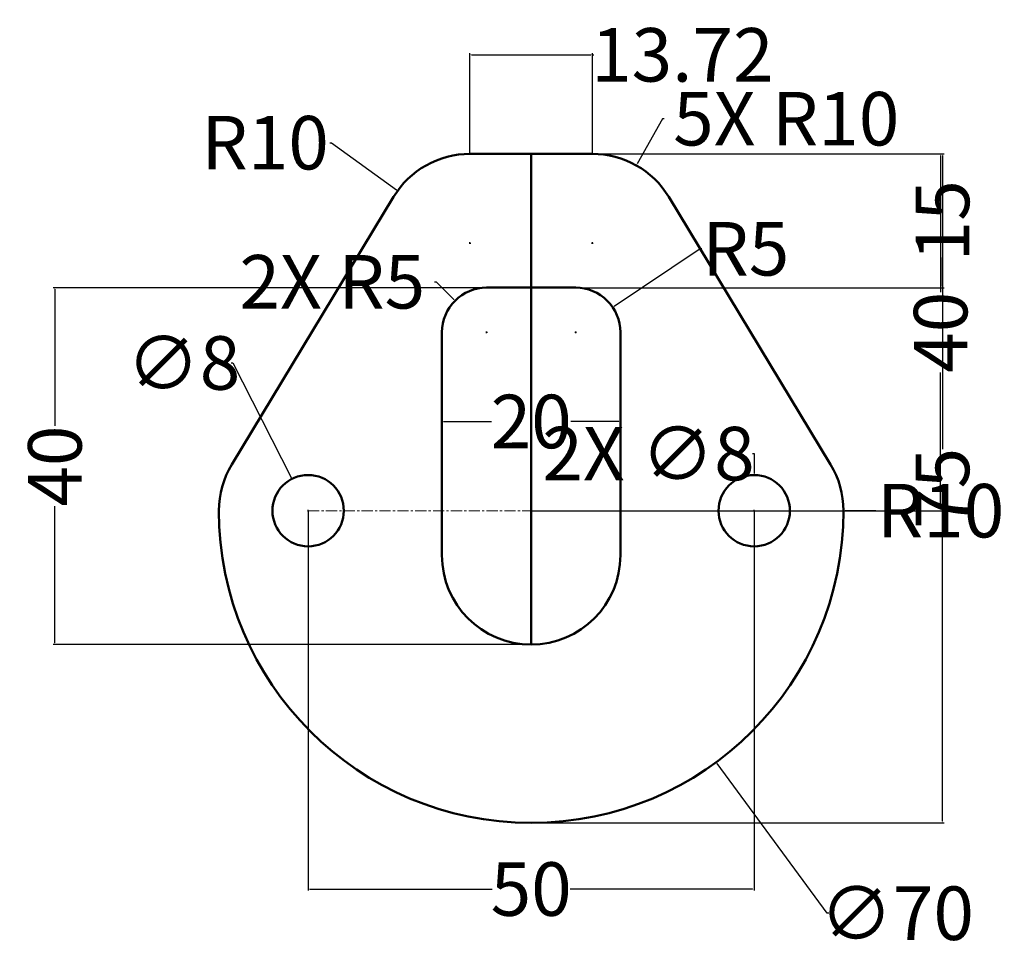
# Model space of a CAD drawing. Units: millimetres. Extents: x 6 to 117, y 2 to 106.
import ezdxf

# ---------------------------------------------------------------- set-up
doc = ezdxf.new("R2010")
doc.units = ezdxf.units.MM
doc.header["$MEASUREMENT"] = 0
doc.linetypes.add('CENTER', pattern=[2, 1.25, -0.25, 0.25, -0.25])
for name, color, linetype, lineweight in [('M-CNTR', 4, 'CENTER', 18), ('M-DIMS', 2, 'Continuous', 25), ('M-OUTL', 7, 'Continuous', 50)]:
    doc.layers.add(name, color=color, linetype=linetype, lineweight=lineweight)
doc.styles.get("Standard").update_dxf_attribs({"font": 'arial.ttf'})
doc.dimstyles.get("Standard").update_dxf_attribs({"dimtxt": 6, "dimasz": 0.18, "dimexe": 0.18, "dimexo": 0.0625, "dimgap": 0.09, "dimtad": 0, "dimtoh": 1, "dimdec": 0, "dimzin": 0, "dimdsep": 46, "dimtxsty": 'Standard', "dimcen": 0.09, "dimadec": 0, "dimazin": 0, "dimtfac": 1, "dimtdec": 0, "dimtofl": 0, "dimtmove": 0, "dimatfit": 3, "dimfxl": 1, "dimtolj": 1, "dimtzin": 0, "dimarcsym": 0})

# ---------------------------------------------------------------- blocks, each defined once
blk = doc.blocks.new('*D1')
at = {"layer": 'Defpoints', "color": 0, "transparency": 16777216}
for p in [(38.77, 50.96), (88.77, 50.96), (88.77, 8.55)]:
    blk.add_point(p, dxfattribs=at)
at = {"layer": 'M-DIMS', "color": 0, "lineweight": -2, "transparency": 16777216}
for p, q in [((38.77, 50.9), (38.77, 8.37)), ((88.77, 50.9), (88.77, 8.37)), ((38.95, 8.55), (59.39, 8.55)), ((88.59, 8.55), (68.15, 8.55))]:
    blk.add_line(p, q, dxfattribs=at)
at = {"layer": 'M-DIMS', "color": 0, "transparency": 16777216}
for points in [[(38.95, 8.58), (38.95, 8.52), (38.77, 8.55)], [(88.59, 8.58), (88.59, 8.52), (88.77, 8.55)]]:
    blk.add_solid(points, dxfattribs=at)
at = {"layer": 'M-DIMS', "color": 0, "transparency": 16777216, "insert": (63.77, 8.55), "char_height": 6, "attachment_point": 5}
blk.add_mtext('\\A1;50', dxfattribs=at)
blk = doc.blocks.new('*D2')
at = {"layer": 'Defpoints', "color": 0, "transparency": 16777216}
for p in [(63.77, 75.96), (10.38, 35.96), (63.77, 35.96)]:
    blk.add_point(p, dxfattribs=at)
at = {"layer": 'M-DIMS', "color": 0, "lineweight": -2, "transparency": 16777216}
for p, q in [((63.71, 75.96), (10.2, 75.96)), ((10.38, 75.78), (10.38, 60.46)), ((10.38, 36.14), (10.38, 51.46)), ((63.71, 35.96), (10.2, 35.96))]:
    blk.add_line(p, q, dxfattribs=at)
at = {"layer": 'M-DIMS', "color": 0, "transparency": 16777216}
for points in [[(10.35, 75.78), (10.41, 75.78), (10.38, 75.96)], [(10.35, 36.14), (10.41, 36.14), (10.38, 35.96)]]:
    blk.add_solid(points, dxfattribs=at)
at = {"layer": 'M-DIMS', "color": 0, "transparency": 16777216, "insert": (10.38, 55.96), "char_height": 6, "attachment_point": 5, "rotation": 90}
blk.add_mtext('\\A1;40', dxfattribs=at)
blk = doc.blocks.new('*D3')
at = {"layer": 'Defpoints', "color": 0, "transparency": 16777216}
for p in [(63.77, 90.96), (109.66, 90.96), (63.77, 50.96)]:
    blk.add_point(p, dxfattribs=at)
at = {"layer": 'M-DIMS', "color": 0, "lineweight": -2, "transparency": 16777216}
for p, q in [((63.83, 90.96), (109.84, 90.96)), ((109.66, 90.78), (109.66, 75.46)), ((109.66, 51.14), (109.66, 66.46)), ((63.83, 50.96), (109.84, 50.96))]:
    blk.add_line(p, q, dxfattribs=at)
at = {"layer": 'M-DIMS', "color": 0, "transparency": 16777216}
for points in [[(109.63, 90.78), (109.69, 90.78), (109.66, 90.96)], [(109.63, 51.14), (109.69, 51.14), (109.66, 50.96)]]:
    blk.add_solid(points, dxfattribs=at)
at = {"layer": 'M-DIMS', "color": 0, "transparency": 16777216, "insert": (109.66, 70.96), "char_height": 6, "attachment_point": 5, "rotation": 90}
blk.add_mtext('\\A1;40', dxfattribs=at)
blk = doc.blocks.new('*D4')
at = {"layer": 'Defpoints', "color": 0, "transparency": 16777216}
for p in [(36.95, 54.52), (40.59, 47.4)]:
    blk.add_point(p, dxfattribs=at)
at = {"layer": 'M-DIMS', "color": 0, "lineweight": -2, "transparency": 16777216}
for p, q in [((30.13, 67.52), (30.31, 67.52)), ((30.31, 67.52), (36.87, 54.68)), ((38.68, 50.96), (38.86, 50.96)), ((38.77, 50.87), (38.77, 51.05))]:
    blk.add_line(p, q, dxfattribs=at)
at = {"layer": 'M-DIMS', "color": 0, "transparency": 16777216}
blk.add_solid([(36.89, 54.7), (36.84, 54.67), (36.95, 54.52)], dxfattribs=at)
at = {"layer": 'M-DIMS', "color": 0, "transparency": 16777216, "insert": (24.8, 67.52), "char_height": 6, "attachment_point": 5}
blk.add_mtext('\\A1;∅8', dxfattribs=at)
blk = doc.blocks.new('*D5')
at = {"layer": 'Defpoints', "color": 0, "transparency": 16777216}
for p in [(88.77, 50.96), (98.77, 50.96)]:
    blk.add_point(p, dxfattribs=at)
at = {"layer": 'M-DIMS', "color": 0, "lineweight": -2, "transparency": 16777216}
for p, q in [((88.68, 50.96), (88.86, 50.96)), ((88.77, 50.87), (88.77, 51.05)), ((102.41, 50.96), (98.95, 50.96))]:
    blk.add_line(p, q, dxfattribs=at)
at = {"layer": 'M-DIMS', "color": 0, "transparency": 16777216}
blk.add_solid([(98.95, 50.99), (98.95, 50.93), (98.77, 50.96)], dxfattribs=at)
at = {"layer": 'M-DIMS', "color": 0, "transparency": 16777216, "insert": (109.66, 50.96), "char_height": 6, "attachment_point": 5}
blk.add_mtext('\\A1;R10', dxfattribs=at)
blk = doc.blocks.new('*D6')
at = {"layer": 'Defpoints', "color": 0, "transparency": 16777216}
for p in [(53.77, 60.96), (73.77, 60.96), (73.77, 60.96)]:
    blk.add_point(p, dxfattribs=at)
at = {"layer": 'M-DIMS', "color": 0, "lineweight": -2, "transparency": 16777216}
for p, q in [((53.77, 61.02), (53.77, 61.14)), ((53.95, 60.96), (59.34, 60.96)), ((73.59, 60.96), (68.2, 60.96)), ((73.77, 61.02), (73.77, 61.14))]:
    blk.add_line(p, q, dxfattribs=at)
at = {"layer": 'M-DIMS', "color": 0, "transparency": 16777216}
for points in [[(53.95, 60.99), (53.95, 60.93), (53.77, 60.96)], [(73.59, 60.99), (73.59, 60.93), (73.77, 60.96)]]:
    blk.add_solid(points, dxfattribs=at)
at = {"layer": 'M-DIMS', "color": 0, "transparency": 16777216, "insert": (63.77, 60.96), "char_height": 6, "attachment_point": 5}
blk.add_mtext('\\A1;20', dxfattribs=at)
blk = doc.blocks.new('*D7')
at = {"layer": 'Defpoints', "color": 0, "transparency": 16777216}
for p in [(72.92, 73.75), (68.77, 70.96)]:
    blk.add_point(p, dxfattribs=at)
at = {"layer": 'M-DIMS', "color": 0, "lineweight": -2, "transparency": 16777216}
for p, q in [((82.7, 80.32), (73.07, 73.85)), ((82.88, 80.32), (82.7, 80.32)), ((68.68, 70.96), (68.86, 70.96)), ((68.77, 70.87), (68.77, 71.05))]:
    blk.add_line(p, q, dxfattribs=at)
at = {"layer": 'M-DIMS', "color": 0, "transparency": 16777216}
blk.add_solid([(73.05, 73.87), (73.09, 73.82), (72.92, 73.75)], dxfattribs=at)
at = {"layer": 'M-DIMS', "color": 0, "transparency": 16777216, "insert": (87.83, 80.32), "char_height": 6, "attachment_point": 5}
blk.add_mtext('\\A1;R5', dxfattribs=at)
blk = doc.blocks.new('*D8')
at = {"layer": 'Defpoints', "color": 0, "transparency": 16777216}
for p in [(48.81, 86.83), (56.91, 80.96)]:
    blk.add_point(p, dxfattribs=at)
at = {"layer": 'M-DIMS', "color": 0, "lineweight": -2, "transparency": 16777216}
for p, q in [((41.2, 92.21), (41.38, 92.21)), ((41.38, 92.21), (48.66, 86.93)), ((56.82, 80.96), (57, 80.96)), ((56.91, 80.87), (56.91, 81.05))]:
    blk.add_line(p, q, dxfattribs=at)
at = {"layer": 'M-DIMS', "color": 0, "transparency": 16777216}
blk.add_solid([(48.68, 86.96), (48.65, 86.91), (48.81, 86.83)], dxfattribs=at)
at = {"layer": 'M-DIMS', "color": 0, "transparency": 16777216, "insert": (33.95, 92.21), "char_height": 6, "attachment_point": 5}
blk.add_mtext('\\A1;R10', dxfattribs=at)
blk = doc.blocks.new('MOUNT-HOLE-D8')
blk.add_circle((4, 4), 4)
blk = doc.blocks.new('*D10')
at = {"layer": 'Defpoints', "color": 0, "transparency": 16777216}
for p in [(70.63, 90.96), (109.87, 90.96), (63.77, 15.96)]:
    blk.add_point(p, dxfattribs=at)
at = {"layer": 'M-DIMS', "color": 0, "lineweight": -2, "transparency": 16777216}
for p, q in [((70.69, 90.96), (110.05, 90.96)), ((109.87, 90.78), (109.87, 57.85)), ((109.87, 16.14), (109.87, 49.08)), ((63.83, 15.96), (110.05, 15.96))]:
    blk.add_line(p, q, dxfattribs=at)
at = {"layer": 'M-DIMS', "color": 0, "transparency": 16777216}
for points in [[(109.84, 90.78), (109.9, 90.78), (109.87, 90.96)], [(109.84, 16.14), (109.9, 16.14), (109.87, 15.96)]]:
    blk.add_solid(points, dxfattribs=at)
at = {"layer": 'M-DIMS', "color": 0, "transparency": 16777216, "insert": (109.87, 53.46), "char_height": 6, "attachment_point": 5, "rotation": 90}
blk.add_mtext('\\A1;75', dxfattribs=at)
blk = doc.blocks.new('*D11')
at = {"layer": 'Defpoints', "color": 0, "transparency": 16777216}
for p in [(70.63, 102.06), (56.91, 90.96), (70.63, 90.96)]:
    blk.add_point(p, dxfattribs=at)
at = {"layer": 'M-DIMS', "color": 0, "lineweight": -2, "transparency": 16777216}
for p, q in [((56.91, 91.02), (56.91, 102.24)), ((57.09, 102.06), (70.45, 102.06)), ((70.63, 91.02), (70.63, 102.24)), ((70.63, 102.06), (70.81, 102.06))]:
    blk.add_line(p, q, dxfattribs=at)
at = {"layer": 'M-DIMS', "color": 0, "transparency": 16777216}
for points in [[(57.09, 102.09), (57.09, 102.03), (56.91, 102.06)], [(70.45, 102.09), (70.45, 102.03), (70.63, 102.06)]]:
    blk.add_solid(points, dxfattribs=at)
at = {"layer": 'M-DIMS', "color": 0, "transparency": 16777216, "insert": (80.71, 102.06), "char_height": 6, "attachment_point": 5}
blk.add_mtext('\\A1;13.72', dxfattribs=at)
blk = doc.blocks.new('*D12')
at = {"layer": 'Defpoints', "color": 0, "transparency": 16777216}
for p in [(70.63, 90.96), (109.87, 90.96), (68.77, 75.96)]:
    blk.add_point(p, dxfattribs=at)
at = {"layer": 'M-DIMS', "color": 0, "lineweight": -2, "transparency": 16777216}
for p, q in [((70.69, 90.96), (110.05, 90.96)), ((109.87, 90.78), (109.87, 87.59)), ((109.87, 76.14), (109.87, 79.33)), ((68.83, 75.96), (110.05, 75.96))]:
    blk.add_line(p, q, dxfattribs=at)
at = {"layer": 'M-DIMS', "color": 0, "transparency": 16777216}
for points in [[(109.84, 90.78), (109.9, 90.78), (109.87, 90.96)], [(109.84, 76.14), (109.9, 76.14), (109.87, 75.96)]]:
    blk.add_solid(points, dxfattribs=at)
at = {"layer": 'M-DIMS', "color": 0, "transparency": 16777216, "insert": (109.87, 83.46), "char_height": 6, "attachment_point": 5, "rotation": 90}
blk.add_mtext('\\A1;15', dxfattribs=at)
blk = doc.blocks.new('*D13')
at = {"layer": 'Defpoints', "color": 0, "transparency": 16777216}
for p in [(88.77, 54.96), (88.77, 46.96)]:
    blk.add_point(p, dxfattribs=at)
at = {"layer": 'M-DIMS', "color": 0, "lineweight": -2, "transparency": 16777216}
for p, q in [((88.59, 57.36), (88.77, 57.36)), ((88.77, 57.36), (88.77, 55.14)), ((88.68, 50.96), (88.86, 50.96)), ((88.77, 50.87), (88.77, 51.05))]:
    blk.add_line(p, q, dxfattribs=at)
at = {"layer": 'M-DIMS', "color": 0, "transparency": 16777216}
blk.add_solid([(88.8, 55.14), (88.74, 55.14), (88.77, 54.96)], dxfattribs=at)
at = {"layer": 'M-DIMS', "color": 0, "transparency": 16777216, "insert": (76.92, 57.36), "char_height": 6, "attachment_point": 5}
blk.add_mtext('\\A1;2X ∅8', dxfattribs=at)
blk = doc.blocks.new('*D14')
at = {"layer": 'Defpoints', "color": 0, "transparency": 16777216}
for p in [(43.04, 79.16), (84.5, 22.76)]:
    blk.add_point(p, dxfattribs=at)
at = {"layer": 'M-DIMS', "color": 0, "lineweight": -2, "transparency": 16777216}
for p, q in [((63.68, 50.96), (63.86, 50.96)), ((63.77, 50.87), (63.77, 51.05)), ((96.94, 5.84), (84.61, 22.62)), ((97.12, 5.84), (96.94, 5.84))]:
    blk.add_line(p, q, dxfattribs=at)
at = {"layer": 'M-DIMS', "color": 0, "transparency": 16777216}
blk.add_solid([(84.63, 22.64), (84.58, 22.6), (84.5, 22.76)], dxfattribs=at)
at = {"layer": 'M-DIMS', "color": 0, "transparency": 16777216, "insert": (104.76, 5.84), "char_height": 6, "attachment_point": 5}
blk.add_mtext('\\A1;∅70', dxfattribs=at)
blk = doc.blocks.new('*D15')
at = {"layer": 'Defpoints', "color": 0, "transparency": 16777216}
for p in [(75.54, 89.67), (70.63, 80.96)]:
    blk.add_point(p, dxfattribs=at)
at = {"layer": 'M-DIMS', "color": 0, "lineweight": -2, "transparency": 16777216}
for p, q in [((78.49, 94.9), (75.63, 89.83)), ((78.67, 94.9), (78.49, 94.9)), ((70.54, 80.96), (70.72, 80.96)), ((70.63, 80.87), (70.63, 81.05))]:
    blk.add_line(p, q, dxfattribs=at)
at = {"layer": 'M-DIMS', "color": 0, "transparency": 16777216}
blk.add_solid([(75.6, 89.84), (75.66, 89.81), (75.54, 89.67)], dxfattribs=at)
at = {"layer": 'M-DIMS', "color": 0, "transparency": 16777216, "insert": (92.36, 94.9), "char_height": 6, "attachment_point": 5}
blk.add_mtext('\\A1;5X R10', dxfattribs=at)
blk = doc.blocks.new('*D16')
at = {"layer": 'Defpoints', "color": 0, "transparency": 16777216}
for p in [(55.23, 74.5), (58.77, 70.96)]:
    blk.add_point(p, dxfattribs=at)
at = {"layer": 'M-DIMS', "color": 0, "lineweight": -2, "transparency": 16777216}
for p, q in [((52.93, 76.62), (53.11, 76.62)), ((53.11, 76.62), (55.11, 74.62)), ((58.68, 70.96), (58.86, 70.96)), ((58.77, 70.87), (58.77, 71.05))]:
    blk.add_line(p, q, dxfattribs=at)
at = {"layer": 'M-DIMS', "color": 0, "transparency": 16777216}
blk.add_solid([(55.13, 74.65), (55.08, 74.6), (55.23, 74.5)], dxfattribs=at)
at = {"layer": 'M-DIMS', "color": 0, "transparency": 16777216, "insert": (41.48, 76.62), "char_height": 6, "attachment_point": 5}
blk.add_mtext('\\A1;2X R5', dxfattribs=at)

msp = doc.modelspace()

# ---------------------------------------------------------------- linework, layer by layer
at = {"layer": 'M-CNTR'}
msp.add_line((38.768, 50.961), (88.768, 50.961), dxfattribs=at)
at = {"layer": 'M-OUTL'}
msp.add_lwpolyline([(63.768, 90.961), (70.629, 90.961, -0.2625357), (79.186, 86.136), (97.326, 56.136, -0.1368013), (98.768, 50.961, -1), (28.768, 50.961, -0.1368013), (30.211, 56.136), (48.351, 86.136, -0.2625357), (56.908, 90.961), (63.768, 90.961), (63.768, 50.961), (63.768, 35.961)], format="xyb", dxfattribs=at)
msp.add_lwpolyline([(58.768, 75.961, 0.4142136), (53.768, 70.961), (53.768, 50.961), (53.768, 45.961, 1), (73.768, 45.961), (73.768, 50.961), (73.768, 70.961, 0.4142136), (68.768, 75.961), (63.768, 75.961)], format="xyb", close=True, dxfattribs=at)

# ---------------------------------------------------------------- block references
for p in [(34.768, 46.961), (84.768, 46.961)]:
    msp.add_blockref('MOUNT-HOLE-D8', p, dxfattribs=at)

# ---------------------------------------------------------------- dimensions: what is measured, and where the dimension line sits
at = {"layer": 'M-DIMS'}
for base, p1, p2, override, picture, middle in [((70.629, 102.061), (56.908, 90.961), (70.629, 90.961), {"dimdec": 2, "dimlfac": 1, "dimrnd": 0, "dimzin": 0, "dimdsep": 46, "dimlunit": 2}, '*D11', (80.709, 102.061)), ((73.768, 60.961), (53.768, 60.961), (73.768, 60.961), {"dimclrd": 0, "dimclre": 0, "dimclrt": 0}, '*D6', (63.768, 60.961)), ((88.768, 8.548), (38.768, 50.961), (88.768, 50.961), {"dimclrd": 0, "dimclre": 0, "dimclrt": 0}, '*D1', (63.768, 8.548))]:
    dim = msp.add_linear_dim(base=base, p1=p1, p2=p2, dimstyle='Standard', override=override, dxfattribs=at)
    dim.commit()
    dim.dimension.update_dxf_attribs({"geometry": picture, "text_midpoint": middle})
for center, mpoint, text, picture, middle in [((70.629, 80.961), (75.541, 89.672), '5X <>', '*D15', (92.362, 94.898)), ((58.768, 70.961), (55.233, 74.497), '2X <>', '*D16', (41.484, 76.618))]:
    dim = msp.add_radius_dim(center=center, mpoint=mpoint, text=text, dimstyle='Standard', override={"dimdec": 0, "dimlfac": 1, "dimrnd": 0, "dimzin": 0, "dimdsep": 46, "dimlunit": 2}, dxfattribs=at)
    dim.commit()
    dim.dimension.update_dxf_attribs({"geometry": picture, "text_midpoint": middle, "dimtype": 164})
for center, mpoint, picture, middle in [((56.908, 80.961), (48.81, 86.829), '*D8', (33.95, 92.214)), ((68.768, 70.961), (72.92, 73.749), '*D7', (87.834, 80.318)), ((88.768, 50.961), (98.768, 50.961), '*D5', (109.658, 50.961))]:
    dim = msp.add_radius_dim(center=center, mpoint=mpoint, dimstyle='Standard', override={"dimclrd": 0, "dimclre": 0, "dimclrt": 0}, dxfattribs=at)
    dim.commit()
    dim.dimension.update_dxf_attribs({"geometry": picture, "text_midpoint": middle, "dimtype": 164})
for base, p1, p2, override, picture, middle in [((109.658, 90.961), (63.768, 50.961), (63.768, 90.961), {"dimclrd": 0, "dimclre": 0, "dimclrt": 0}, '*D3', (109.658, 70.961)), ((109.868, 90.961), (63.768, 15.961), (70.629, 90.961), {"dimdec": 0, "dimlfac": 1, "dimrnd": 0, "dimzin": 0, "dimdsep": 46, "dimlunit": 2}, '*D10', (109.868, 53.461)), ((109.868, 90.961), (68.768, 75.961), (70.629, 90.961), {"dimdec": 0, "dimlfac": 1, "dimrnd": 0, "dimzin": 0, "dimdsep": 46, "dimlunit": 2}, '*D12', (109.868, 83.461)), ((10.376, 35.961), (63.768, 75.961), (63.768, 35.961), {"dimclrd": 0, "dimclre": 0, "dimclrt": 0}, '*D2', (10.376, 55.961))]:
    dim = msp.add_linear_dim(base=base, p1=p1, p2=p2, angle=90, dimstyle='Standard', override=override, dxfattribs=at)
    dim.commit()
    dim.dimension.update_dxf_attribs({"geometry": picture, "text_midpoint": middle})
for p1, p2, override, picture, middle in [((43.035, 79.16), (84.501, 22.763), {"dimdec": 0, "dimlfac": 1, "dimrnd": 0, "dimzin": 0, "dimdsep": 46, "dimlunit": 2}, '*D14', (104.762, 5.844)), ((40.589, 47.4), (36.948, 54.523), {"dimclrd": 0, "dimclre": 0, "dimclrt": 0}, '*D4', (24.799, 67.52))]:
    dim = msp.add_diameter_dim_2p(p1=p1, p2=p2, dimstyle='Standard', override=override, dxfattribs=at)
    dim.commit()
    dim.dimension.update_dxf_attribs({"geometry": picture, "text_midpoint": middle, "dimtype": 163})
dim = msp.add_diameter_dim_2p(p1=(88.769, 46.961), p2=(88.768, 54.961), text='2X <>', dimstyle='Standard', override={"dimdec": 0, "dimlfac": 1, "dimrnd": 0, "dimzin": 0, "dimdsep": 46, "dimlunit": 2}, dxfattribs=at)
dim.commit()
dim.dimension.update_dxf_attribs({"geometry": '*D13', "text_midpoint": (76.923, 57.361), "dimtype": 163})

doc.saveas('drawing.dxf')
